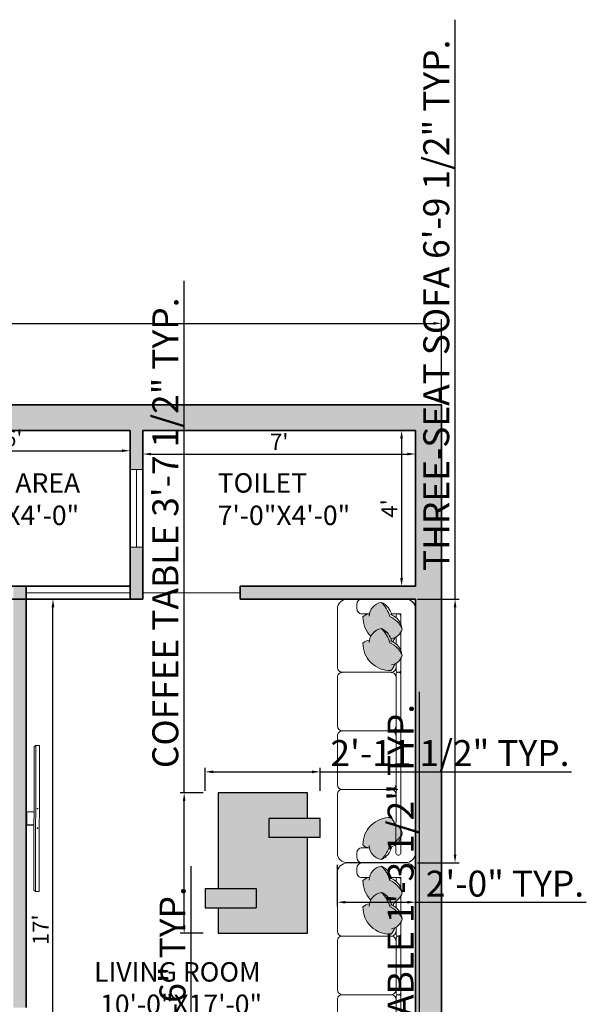
# Model space of a CAD drawing. Units: inches. Extents: x 3259 to 4981, y 1402 to 2026.
# Tile 7 of 11: x 3838 to 4012, y 1722 to 2026. Entities that reach past the tile are written whole.
import ezdxf

# ---------------------------------------------------------------- set-up
doc = ezdxf.new("R2010")
doc.units = ezdxf.units.IN
for name, color, linetype, lineweight in [('A-ANNO-DIMS', 2, 'Continuous', 13), ('A-AREA-IDEN', 7, 'Continuous', 18), ('A-DOOR', 3, 'Continuous', 18), ('A-EQPM', 8, 'Continuous', 18), ('A-FURN', 8, 'Continuous', 13), ('A-GLAZ', 4, 'Continuous', 18), ('A-WALL', 7, 'Continuous', 35), ('A-WALL-PATT', 252, 'Continuous', 13), ('parede', 7, 'Continuous', 30)]:
    doc.layers.add(name, color=color, linetype=linetype, lineweight=lineweight)
doc.styles.get("Standard").update_dxf_attribs({"font": 'arial.ttf'})
doc.dimstyles.new('ISO-25', dxfattribs={"dimtxt": 8, "dimasz": 2.5, "dimexe": 1.25, "dimexo": 0.625, "dimtad": 1, "dimdec": 1, "dimlunit": 3, "dimtxsty": 'Standard', "dimcen": 2.5, "dimclrd": 4, "dimclre": 4, "dimclrt": 1, "dimadec": 0, "dimazin": 0, "dimtfac": 1, "dimtdec": 1, "dimtmove": 0, "dimatfit": 3, "dimfxl": 1, "dimarcsym": 0})

# ---------------------------------------------------------------- blocks, each defined once
blk = doc.blocks.new('SOFA 1')
at = {"transparency": 33554687}
h = blk.add_hatch(color=256, dxfattribs=at)
h.dxf.hatch_style = 1
h.paths.add_polyline_path([(3723.52, 1308.63, 0.147724), (3717.76, 1305.24, 0.310469), (3722.42, 1300.4), (3722.42, 1300.25, 0.156703), (3723.62, 1297.8, 0.425821), (3734.69, 1309.08, 0.121928), (3732.05, 1310.63, 0.233216), (3728.6, 1313.59, 0.213835)])
h = blk.add_hatch(color=256, dxfattribs=at)
h.dxf.hatch_style = 1
h.paths.add_polyline_path([(3769.65, 1307.6, 0.084911), (3767.15, 1309.12, 0.046133), (3766.46, 1311.13), (3759.18, 1311.13, 0.039409), (3758.92, 1310.24, 0.165523), (3756.31, 1309.02, 0.42585), (3767.59, 1297.95, 0.121928), (3769.15, 1300.58, 0.027403), (3769.65, 1300.83)])
h.paths.add_polyline_path([(3765.34, 1313.08), (3760.4, 1313.08, 0.097704), (3759.18, 1311.13), (3766.46, 1311.13, 0.04873)])
h.paths.add_polyline_path([(3763.76, 1314.88, 0.16488), (3760.4, 1313.08), (3765.34, 1313.08, 0.051917)])
h.paths.add_polyline_path([(3771.6, 1305.17, 0.090388), (3769.65, 1307.6), (3769.65, 1300.83, 0.136035), (3771.6, 1302.77)])
h = blk.add_hatch(color=256, dxfattribs=at)
h.dxf.hatch_style = 1
h.paths.add_polyline_path([(3769.16, 1235.96, 0.122267), (3767.6, 1238.61, 0.425972), (3756.32, 1227.54, 0.165563), (3758.93, 1226.32, 0.309481), (3763.76, 1221.69, 0.002677), (3763.83, 1221.72, 0.146094), (3767.16, 1227.43, 0.212433), (3772.1, 1232.48, 0.235342)])
h = blk.add_hatch(color=256, dxfattribs=at)
h.dxf.hatch_style = 1
h.paths.add_polyline_path([(3769.16, 1225.36, 0.122267), (3767.6, 1228.01, 0.425972), (3756.32, 1216.94, 0.165563), (3758.93, 1215.72, 0.309481), (3763.76, 1211.09, 0.002677), (3763.83, 1211.12, 0.146094), (3767.16, 1216.83, 0.212433), (3772.1, 1221.88, 0.235342)])
for p, q in [((3720.45, 1316.13), (3773.58, 1316.13)), ((3777.51, 1312.19), (3777.51, 1213.72))]:
    blk.add_line(p, q, dxfattribs=at)
for points in [[(3716.51, 1312.2), (3716.51, 1291.44)], [(3722.42, 1313.08), (3722.42, 1309.23), (3722.42, 1313.08), (3726.57, 1313.08)], [(3729.85, 1313.08), (3745.25, 1313.08)], [(3746.01, 1312.3), (3746.01, 1288.55)], [(3768.11, 1313.08), (3746.78, 1313.08)], [(3771.6, 1313.08), (3767.75, 1313.08), (3771.6, 1313.08), (3771.6, 1308.93)], [(3769.66, 1287.39), (3769.65, 1312.3)], [(3771.6, 1313.08), (3771.61, 1233.74)], [(3723.21, 1311.13), (3723.93, 1311.13)], [(3731.82, 1311.13), (3745.25, 1311.13)], [(3746.01, 1310.97), (3746.01, 1311.36)], [(3746.01, 1288.54), (3746.01, 1308.23)], [(3768.87, 1311.13), (3746.78, 1311.13)], [(3769.65, 1309.43), (3769.65, 1308.71)], [(3722.42, 1300.39), (3722.42, 1297.33)], [(3720.45, 1295.38), (3718.48, 1295.38)], [(3720.45, 1287.5), (3744.09, 1287.5)], [(3746.02, 1284.63), (3746.02, 1264.94)], [(3747.99, 1286.6), (3767.69, 1286.6)], [(3769.66, 1263.75), (3769.66, 1285.81)], [(3769.66, 1277.18), (3769.66, 1263.75)], [(3746.02, 1260.99), (3746.02, 1241.3)], [(3747.99, 1262.97), (3767.69, 1262.97)], [(3769.66, 1240.12), (3769.66, 1262.18)], [(3770.43, 1262.97), (3770.82, 1262.97)], [(3746.02, 1237.36), (3746.02, 1213.74)], [(3747.99, 1239.33), (3767.69, 1239.33)], [(3769.66, 1235.71), (3769.66, 1238.54)], [(3770.43, 1239.33), (3770.82, 1239.33)], [(3771.61, 1223.14), (3771.61, 1230.47)], [(3769.66, 1225.11), (3769.66, 1227.82)], [(3767.76, 1215.72), (3771.61, 1215.72), (3771.61, 1219.84), (3771.61, 1215.72)], [(3769.66, 1216.5), (3769.66, 1217.22)], [(3753.91, 1211.77), (3753.91, 1213.74)], [(3755.86, 1215.72), (3758.92, 1215.72)], [(3749.97, 1209.8), (3773.58, 1209.8)]]:
    blk.add_lwpolyline(points, close=True, dxfattribs=at)
for points in [[(3717.76, 1305.24, -0.147724), (3723.52, 1308.63, -0.213355), (3728.59, 1313.59, 0.213355), (3723.52, 1308.63, 0.147724), (3717.76, 1305.24, -0.249545), (3722.86, 1309.34, 0.249545), (3717.75, 1305.25, 0.356779), (3723.4, 1300.28, -0.356779), (3717.76, 1305.24)], [(3728.58, 1313.6, -0.306333), (3732.42, 1309.31, 0.306333), (3728.58, 1313.6, 0.306674), (3722.72, 1308.89, -0.306674), (3728.58, 1313.6)], [(3763.76, 1314.88, -0.147724), (3767.15, 1309.12, -0.213355), (3772.1, 1304.05, 0.213355), (3767.15, 1309.12, 0.147724), (3763.76, 1314.88, -0.249545), (3767.86, 1309.77, 0.249545), (3763.77, 1314.89, 0.356779), (3758.8, 1309.23, -0.356779), (3763.76, 1314.88)], [(3734.69, 1309.08, -0.425972), (3723.62, 1297.8, -0.165552), (3722.4, 1300.4, 0.165552), (3723.62, 1297.79, 0.425972), (3734.69, 1309.07, 0.121514), (3732.07, 1310.63, -0.121514), (3734.69, 1309.08)], [(3767.6, 1297.95, -0.425972), (3756.31, 1309.01, -0.165552), (3758.92, 1310.24, 0.165552), (3756.31, 1309.02, 0.425972), (3767.59, 1297.95, 0.121514), (3769.14, 1300.57, -0.121514), (3767.6, 1297.95)], [(3772.11, 1304.06, -0.306333), (3767.83, 1300.22, 0.306333), (3772.11, 1304.06, 0.306674), (3767.4, 1309.91, -0.306674), (3772.11, 1304.06)], [(3770.44, 1286.63, -0.414214), (3769.66, 1287.4, 0.414214), (3770.44, 1286.63, 0.414214), (3769.66, 1285.83, -0.414214), (3770.44, 1286.63)], [(3748.01, 1262.99, -0.414214), (3746.05, 1264.95, 0.414214), (3748.01, 1262.97, 0.414213), (3746.05, 1261.01, -0.414213), (3748.01, 1262.99)], [(3770.44, 1262.99, -0.414214), (3769.66, 1263.77, 0.414214), (3770.44, 1262.99, 0.414214), (3769.66, 1262.19, -0.414214), (3770.44, 1262.99)], [(3770.83, 1262.97, -0.414214), (3771.61, 1262.19, 0.414214), (3770.83, 1262.99, 0.414214), (3771.61, 1263.77, -0.414214), (3770.83, 1262.97)], [(3748.01, 1239.35, -0.414214), (3746.05, 1241.31, 0.414214), (3748.01, 1239.33, 0.414213), (3746.05, 1237.37, -0.414213), (3748.01, 1239.35)], [(3767.7, 1239.33, -0.414214), (3769.66, 1237.37, 0.414214), (3767.7, 1239.35, 0.414214), (3769.66, 1241.31, -0.414214), (3767.7, 1239.33)], [(3770.44, 1239.35, -0.414214), (3769.66, 1240.13, 0.414214), (3770.44, 1239.33, 0.414214), (3769.66, 1238.55, -0.414214), (3770.44, 1239.35)], [(3770.83, 1239.33, -0.414214), (3771.61, 1238.55, 0.414214), (3770.83, 1239.35, 0.414214), (3771.61, 1240.13, -0.414214), (3770.83, 1239.33)], [(3756.32, 1227.54, -0.425972), (3767.6, 1238.61, -0.121514), (3769.16, 1235.98, 0.121514), (3767.6, 1238.61, 0.425972), (3756.32, 1227.54, 0.165552), (3758.93, 1226.32, -0.165552), (3756.32, 1227.54)], [(3772.1, 1232.5, -0.306674), (3767.41, 1226.64, 0.306674), (3772.1, 1232.5, 0.306333), (3767.84, 1236.34, -0.306333), (3772.1, 1232.5)], [(3763.78, 1221.67, 0.249545), (3767.87, 1226.78, -0.249545), (3763.76, 1221.69, -0.356779), (3758.81, 1227.32, 0.356779), (3763.77, 1221.68, 0.147724), (3767.16, 1227.43, 0.213355), (3772.11, 1232.51, -0.213355), (3767.16, 1227.43, -0.147724), (3763.78, 1221.67)], [(3756.32, 1216.94, -0.200233), (3759.49, 1224.76, 0.200233), (3756.32, 1216.94, 0.165552), (3758.93, 1215.72, -0.165552), (3756.32, 1216.94)], [(3772.1, 1221.9, -0.306674), (3767.41, 1216.04, 0.306674), (3772.1, 1221.9, -0.213355), (3767.16, 1216.83, -0.147724), (3763.77, 1211.08, 0.147724), (3767.15, 1216.83, 0.213355), (3772.1, 1221.9)], [(3763.76, 1211.09, -0.356779), (3758.81, 1216.72, 0.356779), (3763.76, 1211.09, 0.249545), (3767.87, 1216.18, -0.249545), (3763.76, 1211.09)]]:
    blk.add_lwpolyline(points, format="xyb", dxfattribs=at)
for points in [[(3722.42, 1311.91, 0.414214), (3723.2, 1311.13, -0.414214)], [(3770.43, 1313.08, 0.414214), (3769.65, 1312.3, -0.414214)], [(3771.6, 1312.3, 0.414214), (3770.82, 1313.08, -0.414214)], [(3716.51, 1297.34, 0.414214), (3718.47, 1295.38, -0.414214)], [(3720.44, 1295.38, 0.414214), (3722.4, 1297.34, -0.414214)], [(3716.51, 1291.45, 0.414212), (3720.44, 1287.52, -0.414212)], [(3746.03, 1288.56, 0.414214), (3747.99, 1286.6, 0.414213), (3746.03, 1284.64, -0.414213), (3747.99, 1286.6, -0.414214)], [(3769.66, 1284.64, 0.414214), (3767.7, 1286.6, 0.414214), (3769.66, 1288.56, -0.414214), (3767.7, 1286.6, -0.414214)], [(3769.66, 1261.01, 0.414214), (3767.7, 1262.97, 0.414214), (3769.66, 1264.93, -0.414214), (3767.7, 1262.97, -0.414214)], [(3772.13, 1221.9, 0.306333), (3767.84, 1225.74, -0.306333)], [(3769.16, 1225.36, 0.071861), (3768.39, 1227.01, -0.071861)], [(3769.66, 1216.52, 0.414214), (3770.44, 1215.74, -0.414214)], [(3770.83, 1215.74, 0.414214), (3771.61, 1216.52, -0.414214)], [(3746.05, 1213.76, 0.414212), (3749.98, 1209.82, -0.414212)], [(3755.87, 1215.72, 0.414214), (3753.91, 1213.76, -0.414214)], [(3755.87, 1209.8, -0.414214), (3753.91, 1211.76, 0.414214)]]:
    blk.add_lwpolyline(points, format="xyb", close=True, dxfattribs=at)
for centre, radius, start, end in [((3720.44, 1312.2), 3.93, 90.0002, 179.9998), ((3720.44, 1312.19), 3.94, 89.9158, 179.9154), ((3773.58, 1312.2), 3.93, 0.0002, 89.9998), ((3773.57, 1312.19), 3.94, 359.9158, 89.9154), ((3745.22, 1312.29), 0.789, 0.8425, 90.8425), ((3745.24, 1311.91), 0.777, 270, 0), ((3745.24, 1311.91), 0.777, 270, 0), ((3746.8, 1312.29), 0.789, 89.1575, 179.1575), ((3746.79, 1311.91), 0.777, 180, 270), ((3746.79, 1311.91), 0.777, 180, 270), ((3768.87, 1312.3), 0.777, 360, 90), ((3768.87, 1311.91), 0.777, 270, 0), ((3744.09, 1309.21), 1.92, 358.766, 90.5111), ((3747.93, 1309.21), 1.92, 89.4889, 181.234), ((3744.08, 1289.48), 1.96, 270, 360), ((3744.08, 1289.48), 1.96, 270, 360), ((3773.58, 1213.73), 3.93, 270.0002, 359.9998), ((3773.59, 1213.73), 3.93, 269.9156, 359.9152)]:
    blk.add_arc(centre, radius, start, end, dxfattribs=at)
blk = doc.blocks.new('Mesa de Centro Nalita')
at = {"layer": 'parede', "ltscale": 0.2}
h = blk.add_hatch(color=256, dxfattribs=at)
h.set_gradient(color1=(95, 72, 63), color2=(161, 128, 114), one_color=1, tint=0.54, name='INVCYLINDER')
h.paths.add_polyline_path([(0.35, -0.35), (0.05, -0.35), (0.05, -0.2), (0.35, -0.2), (0.35, 0), (-0.35, 0), (-0.35, -0.75), (-0.05, -0.75), (-0.05, -0.9), (-0.35, -0.9), (-0.35, -1.1), (0.35, -1.1)])
h = blk.add_hatch(color=256, dxfattribs=at)
h.set_gradient(color1=(95, 72, 63), color2=(161, 128, 114), one_color=1, tint=0.54, name='INVSPHERICAL')
h.paths.add_polyline_path([(0.05, -0.2), (0.05, -0.35), (0.45, -0.35), (0.45, -0.2)])
h = blk.add_hatch(color=256, dxfattribs=at)
h.set_gradient(color1=(95, 72, 63), color2=(161, 128, 114), one_color=1, tint=0.54, name='INVSPHERICAL')
h.paths.add_polyline_path([(-0.05, -0.9), (-0.05, -0.75), (-0.45, -0.75), (-0.45, -0.9)])
for p, q in [((0.35, 0), (-0.35, 0)), ((-0.35, 0), (-0.35, -0.75)), ((0.35, -0.2), (0.35, 0)), ((0.05, -0.35), (0.05, -0.2)), ((0.45, -0.2), (0.05, -0.2)), ((0.45, -0.35), (0.45, -0.2)), ((0.45, -0.35), (0.05, -0.35)), ((0.35, -1.1), (0.35, -0.35)), ((-0.45, -0.75), (-0.05, -0.75)), ((-0.45, -0.75), (-0.45, -0.9)), ((-0.05, -0.75), (-0.05, -0.9)), ((-0.45, -0.9), (-0.05, -0.9)), ((-0.35, -0.9), (-0.35, -1.1)), ((-0.35, -1.1), (0.35, -1.1))]:
    blk.add_line(p, q, dxfattribs=at)
blk = doc.blocks.new('*D44')
at = {"layer": 'A-ANNO-DIMS', "color": 0, "lineweight": -2, "transparency": 16777216}
for p, q in [((3799.66, 1898.49), (3799.66, 1891.66)), ((3871.66, 1898.49), (3871.66, 1891.66)), ((3802.16, 1892.91), (3869.16, 1892.91))]:
    blk.add_line(p, q, dxfattribs=at)
at = {"layer": 'A-ANNO-DIMS', "color": 0, "transparency": 16777216}
for points in [[(3802.16, 1893.33), (3802.16, 1892.5), (3799.66, 1892.91)], [(3869.16, 1893.33), (3869.16, 1892.5), (3871.66, 1892.91)]]:
    blk.add_solid(points, dxfattribs=at)
at = {"layer": 'Defpoints', "color": 0, "transparency": 16777216}
for p in [(3799.66, 1899.12), (3871.66, 1899.12), (3871.66, 1892.91)]:
    blk.add_point(p, dxfattribs=at)
at = {"layer": 'A-ANNO-DIMS', "color": 0, "transparency": 16777216, "insert": (3835.66, 1896.09), "char_height": 5, "attachment_point": 5}
blk.add_mtext("6'", dxfattribs=at)
blk = doc.blocks.new('*D45')
at = {"layer": 'A-ANNO-DIMS', "color": 0, "lineweight": -2, "transparency": 16777216}
for p, q in [((3875.66, 1898.49), (3875.66, 1890.65)), ((3959.66, 1898.49), (3959.66, 1890.65)), ((3878.16, 1891.9), (3957.16, 1891.9))]:
    blk.add_line(p, q, dxfattribs=at)
at = {"layer": 'A-ANNO-DIMS', "color": 0, "transparency": 16777216}
for points in [[(3878.16, 1892.31), (3878.16, 1891.48), (3875.66, 1891.9)], [(3957.16, 1892.31), (3957.16, 1891.48), (3959.66, 1891.9)]]:
    blk.add_solid(points, dxfattribs=at)
at = {"layer": 'Defpoints', "color": 0, "transparency": 16777216}
for p in [(3875.66, 1899.12), (3959.66, 1899.12), (3959.66, 1891.9)]:
    blk.add_point(p, dxfattribs=at)
at = {"layer": 'A-ANNO-DIMS', "color": 0, "transparency": 16777216, "insert": (3917.66, 1895.02), "char_height": 5, "attachment_point": 5}
blk.add_mtext("7'", dxfattribs=at)
blk = doc.blocks.new('*D46')
at = {"layer": 'A-ANNO-DIMS', "color": 0, "lineweight": -2, "transparency": 16777216}
for p, q in [((3959.04, 1899.12), (3954.13, 1899.12)), ((3955.38, 1896.62), (3955.38, 1853.62)), ((3959.04, 1851.12), (3954.13, 1851.12))]:
    blk.add_line(p, q, dxfattribs=at)
at = {"layer": 'A-ANNO-DIMS', "color": 0, "transparency": 16777216}
for points in [[(3954.96, 1896.62), (3955.79, 1896.62), (3955.38, 1899.12)], [(3954.96, 1853.62), (3955.79, 1853.62), (3955.38, 1851.12)]]:
    blk.add_solid(points, dxfattribs=at)
at = {"layer": 'Defpoints', "color": 0, "transparency": 16777216}
for p in [(3959.66, 1899.12), (3955.38, 1851.12), (3959.66, 1851.12)]:
    blk.add_point(p, dxfattribs=at)
at = {"layer": 'A-ANNO-DIMS', "color": 0, "transparency": 16777216, "insert": (3952.25, 1875.12), "char_height": 5, "attachment_point": 5, "rotation": 90}
blk.add_mtext("4'", dxfattribs=at)
blk = doc.blocks.new('*D56')
at = {"layer": 'A-ANNO-DIMS', "color": 0, "lineweight": -2, "transparency": 16777216}
for p, q in [((3840.29, 1847.12), (3849.16, 1847.12)), ((3847.91, 1645.62), (3847.91, 1844.62)), ((3840.29, 1643.12), (3849.16, 1643.12))]:
    blk.add_line(p, q, dxfattribs=at)
at = {"layer": 'A-ANNO-DIMS', "color": 0, "transparency": 16777216}
for points in [[(3847.49, 1844.62), (3848.33, 1844.62), (3847.91, 1847.12)], [(3847.49, 1645.62), (3848.33, 1645.62), (3847.91, 1643.12)]]:
    blk.add_solid(points, dxfattribs=at)
at = {"layer": 'Defpoints', "color": 0, "transparency": 16777216}
for p in [(3839.66, 1847.12), (3847.91, 1847.12), (3839.66, 1643.12)]:
    blk.add_point(p, dxfattribs=at)
at = {"layer": 'A-ANNO-DIMS', "color": 0, "transparency": 16777216, "insert": (3844.77, 1745.12), "char_height": 5, "attachment_point": 5, "rotation": 90}
blk.add_mtext("17'", dxfattribs=at)
blk = doc.blocks.new('SOFA-3SEAT')
at = {"transparency": 33554687}
h = blk.add_hatch(color=256, dxfattribs=at)
h.dxf.hatch_style = 1
h.paths.add_polyline_path([(17.7, 69.38, -0.122267), (16.5, 67.36, -0.425972), (7.88, 75.82, -0.165563), (9.87, 76.76, -0.309481), (13.57, 80.3, -0.002677), (13.62, 80.27, -0.146094), (16.16, 75.9, -0.212433), (19.95, 72.05, -0.235342)])
h = blk.add_hatch(color=256, dxfattribs=at)
h.dxf.hatch_style = 1
h.paths.add_polyline_path([(17.7, 61.28, -0.122267), (16.5, 59.26, -0.425972), (7.88, 67.72, -0.165563), (9.87, 68.65, -0.309481), (13.57, 72.19, -0.002677), (13.62, 72.17, -0.146094), (16.16, 67.8, -0.212433), (19.95, 63.95, -0.235342)])
h = blk.add_hatch(color=256, dxfattribs=at)
h.dxf.hatch_style = 1
h.paths.add_polyline_path([(18.07, 6.52, -0.084911), (16.16, 5.36, -0.046133), (15.63, 3.82), (10.07, 3.82, -0.039409), (9.87, 4.51, -0.165523), (7.87, 5.44, -0.42585), (16.5, 13.9, -0.121928), (17.69, 11.88, -0.027403), (18.07, 11.69)])
h.paths.add_polyline_path([(14.77, 2.33), (11, 2.33, -0.097704), (10.07, 3.82), (15.63, 3.82, -0.04873)])
h.paths.add_polyline_path([(13.57, 0.96, -0.16488), (11, 2.33), (14.77, 2.33, -0.051917)])
h.paths.add_polyline_path([(19.56, 8.38, -0.090388), (18.07, 6.52), (18.07, 11.69, -0.136035), (19.56, 10.21)])
blk.add_line((24.08, 3.01), (24.08, 78.28), dxfattribs=at)
blk.add_line((18.66, 2.33), (18.96, 2.33))
for points in [[(0.03, 78.26, -0.414212), (3.03, 81.26, 0.414212)], [(7.54, 81.28, 0.414214), (6.04, 79.78, -0.414214)], [(7.54, 76.76, -0.414214), (6.04, 78.26, 0.414214)], [(18.08, 76.15, -0.414214), (18.67, 76.74, 0.414214)], [(18.97, 76.74, -0.414214), (19.57, 76.15, 0.414214)], [(19.96, 72.03, -0.306333), (16.68, 69.1, 0.306333)], [(17.69, 69.39, -0.071861), (17.1, 68.12, 0.071861)], [(18.08, 42.14, -0.414214), (16.58, 40.64, -0.414214), (18.08, 39.14, 0.414214), (16.58, 40.64, 0.414214)], [(0.02, 21.07, -0.414214), (1.52, 22.57, -0.414213), (0.02, 24.07, 0.414213), (1.52, 22.57, 0.414214)], [(18.08, 24.07, -0.414214), (16.58, 22.57, -0.414214), (18.08, 21.07, 0.414214), (16.58, 22.57, 0.414214)], [(7.54, 4.54, 0.414214), (6.04, 3.04, -0.414214)], [(0, 2.93, 0.439287), (3.02, 0.02, -0.439287)], [(7.54, 0.02, -0.414214), (6.04, 1.52, 0.414214)], [(18.66, 2.33, -0.414214), (18.07, 2.93, 0.414214)], [(19.56, 2.93, -0.414214), (18.96, 2.33, 0.414214)]]:
    blk.add_lwpolyline(points, format="xyb", close=True, dxfattribs=at)
for points in [[(3.02, 81.28), (21.07, 81.28)], [(6.04, 79.77), (6.04, 78.27)], [(0.01, 60.21), (0.01, 78.27)], [(7.53, 76.76), (9.87, 76.76)], [(16.62, 76.76), (19.57, 76.76), (19.57, 73.6), (19.57, 76.76)], [(18.08, 76.16), (18.08, 75.61)], [(19.57, 71.08), (19.57, 65.48)], [(18.08, 69.58), (18.08, 67.5)], [(18.08, 61.47), (18.08, 59.31)], [(19.56, 2.93), (19.57, 62.98)], [(1.52, 58.71), (16.57, 58.71)], [(18.08, 58.1), (18.08, 41.24)], [(18.66, 58.71), (18.96, 58.71)], [(0.01, 42.15), (0.01, 57.2)], [(1.52, 40.64), (16.57, 40.64)], [(18.08, 29.77), (18.08, 40.04)], [(18.08, 40.04), (18.08, 23.17)], [(18.66, 40.64), (18.96, 40.64)], [(0.01, 24.08), (0.01, 39.13)], [(1.52, 22.57), (16.57, 22.57)], [(18.08, 21.97), (18.07, 2.93)], [(0, 2.93), (0, 21.08)], [(0, 3.95), (0, 3.64)], [(7.53, 4.54), (9.87, 4.54)], [(18.07, 5.12), (18.07, 5.67)], [(3.02, 0.02), (21.07, 0.02)], [(6.04, 1.52), (6.04, 3.03)]]:
    blk.add_lwpolyline(points, close=True, dxfattribs=at)
for points in [[(13.57, 80.3, 0.356779), (9.78, 75.99, -0.356779), (13.57, 80.3, -0.249545), (16.71, 76.4, 0.249545), (13.57, 80.3)], [(19.94, 72.03, 0.306674), (16.36, 76.51, -0.306674), (19.94, 72.03, 0.213355), (16.16, 75.9, 0.147724), (13.58, 80.3, -0.147724), (16.16, 75.91, -0.213355), (19.94, 72.03)], [(7.88, 75.82, 0.200233), (10.31, 69.84, -0.200233), (7.88, 75.82, -0.165552), (9.87, 76.76, 0.165552), (7.88, 75.82)], [(13.58, 72.21, -0.249545), (16.71, 68.3, 0.249545), (13.57, 72.19, 0.356779), (9.78, 67.89, -0.356779), (13.58, 72.2, -0.147724), (16.16, 67.8, -0.213355), (19.95, 63.92, 0.213355), (16.16, 67.8, 0.147724), (13.58, 72.21)], [(7.88, 67.72, 0.425972), (16.5, 59.26, 0.121514), (17.69, 61.27, -0.121514), (16.5, 59.26, -0.425972), (7.88, 67.72, -0.165552), (9.87, 68.65, 0.165552), (7.88, 67.72)], [(19.94, 63.93, 0.306674), (16.36, 68.41, -0.306674), (19.94, 63.93, -0.306333), (16.68, 61, 0.306333), (19.94, 63.93)], [(1.52, 58.69, 0.414214), (0.03, 57.19, -0.414214), (1.52, 58.71, -0.414213), (0.03, 60.21, 0.414213), (1.52, 58.69)], [(16.58, 58.71, 0.414214), (18.08, 60.21, -0.414214), (16.58, 58.69, -0.414214), (18.08, 57.19, 0.414214), (16.58, 58.71)], [(18.67, 58.69, 0.414214), (18.08, 58.1, -0.414214), (18.67, 58.71, -0.414214), (18.08, 59.3, 0.414214), (18.67, 58.69)], [(18.97, 58.71, 0.414214), (19.57, 59.3, -0.414214), (18.97, 58.69, -0.414214), (19.57, 58.1, 0.414214), (18.97, 58.71)], [(1.52, 40.62, 0.414214), (0.03, 39.12, -0.414214), (1.52, 40.64, -0.414213), (0.03, 42.14, 0.414213), (1.52, 40.62)], [(18.67, 40.62, 0.414214), (18.08, 40.03, -0.414214), (18.67, 40.62, -0.414214), (18.08, 41.23, 0.414214), (18.67, 40.62)], [(18.97, 40.64, 0.414214), (19.57, 41.23, -0.414214), (18.97, 40.62, -0.414214), (19.57, 40.03, 0.414214), (18.97, 40.64)], [(18.67, 22.55, 0.414214), (18.08, 21.96, -0.414214), (18.67, 22.55, -0.414214), (18.08, 23.17, 0.414214), (18.67, 22.55)], [(16.5, 13.9, 0.425972), (7.87, 5.44, 0.165552), (9.87, 4.51, -0.165552), (7.87, 5.44, -0.425972), (16.5, 13.9, -0.121514), (17.68, 11.89, 0.121514), (16.5, 13.9)], [(19.95, 9.23, 0.306333), (16.68, 12.16, -0.306333), (19.95, 9.23, -0.306674), (16.35, 4.75, 0.306674), (19.95, 9.23)], [(13.57, 0.96, 0.147724), (16.16, 5.36, 0.213355), (19.94, 9.23, -0.213355), (16.16, 5.36, -0.147724), (13.57, 0.96, 0.249545), (16.7, 4.86, -0.249545), (13.57, 0.95, -0.356779), (9.77, 5.27, 0.356779), (13.57, 0.96)]]:
    blk.add_lwpolyline(points, format="xyb", dxfattribs=at)
for centre, radius, start, end in [((21.08, 78.28), 3, 0.0848, 90.0844), ((21.07, 78.27), 3.01, 0.0002, 89.9998), ((21.07, 3.01), 3.01, 270.0002, 359.9998), ((21.07, 3.01), 3.01, 270.0846, 0.0842)]:
    blk.add_arc(centre, radius, start, end, dxfattribs=at)
blk = doc.blocks.new('*D152')
at = {"layer": 'A-ANNO-DIMS', "color": 4, "lineweight": -2, "transparency": 16777216}
for p, q in [((3890.55, 1617.63), (3890.55, 1764.73)), ((3886.68, 1617.63), (3891.8, 1617.63)), ((3890.55, 1590.15), (3890.55, 1615.13)), ((3886.68, 1587.65), (3891.8, 1587.65))]:
    blk.add_line(p, q, dxfattribs=at)
at = {"layer": 'A-ANNO-DIMS', "color": 4, "transparency": 16777216}
for points in [[(3890.13, 1615.13), (3890.96, 1615.13), (3890.55, 1617.63)], [(3890.13, 1590.15), (3890.96, 1590.15), (3890.55, 1587.65)]]:
    blk.add_solid(points, dxfattribs=at)
at = {"layer": 'Defpoints', "color": 0, "transparency": 16777216}
for p in [(3886.05, 1617.63), (3890.55, 1617.63), (3886.05, 1587.65)]:
    blk.add_point(p, dxfattribs=at)
at = {"layer": 'A-ANNO-DIMS', "color": 1, "transparency": 16777216, "insert": (3885.79, 1692.43), "char_height": 8, "attachment_point": 5, "rotation": 90}
blk.add_mtext('TERRACE CHAIR 2\'-6" TYP.', dxfattribs=at)
blk = doc.blocks.new('*D160')
at = {"layer": 'A-ANNO-DIMS', "color": 4, "lineweight": -2, "transparency": 16777216}
for p, q in [((3960.87, 1679.69), (3960.87, 1818.51)), ((3959.13, 1679.69), (3962.12, 1679.69)), ((3960.87, 1666.44), (3960.87, 1677.19)), ((3959.13, 1663.94), (3962.12, 1663.94))]:
    blk.add_line(p, q, dxfattribs=at)
at = {"layer": 'A-ANNO-DIMS', "color": 4, "transparency": 16777216}
for points in [[(3960.45, 1677.19), (3961.28, 1677.19), (3960.87, 1679.69)], [(3960.45, 1666.44), (3961.28, 1666.44), (3960.87, 1663.94)]]:
    blk.add_solid(points, dxfattribs=at)
at = {"layer": 'Defpoints', "color": 0, "transparency": 16777216}
for p in [(3958.51, 1679.69), (3960.87, 1679.69), (3958.51, 1663.94)]:
    blk.add_point(p, dxfattribs=at)
at = {"layer": 'A-ANNO-DIMS', "color": 1, "transparency": 16777216, "insert": (3956.1, 1750.35), "char_height": 8, "attachment_point": 5, "rotation": 90}
blk.add_mtext('SIDE TABLE 1\'-3 1/2" TYP.', dxfattribs=at)
blk = doc.blocks.new('*D162')
at = {"layer": 'A-ANNO-DIMS', "color": 4, "lineweight": -2, "transparency": 16777216}
for p, q in [((3888.35, 1787.34), (3888.35, 1945.34)), ((3894.22, 1787.34), (3887.1, 1787.34)), ((3888.35, 1746.53), (3888.35, 1784.84)), ((3894.22, 1744.03), (3887.1, 1744.03))]:
    blk.add_line(p, q, dxfattribs=at)
at = {"layer": 'A-ANNO-DIMS', "color": 4, "transparency": 16777216}
for points in [[(3887.94, 1784.84), (3888.77, 1784.84), (3888.35, 1787.34)], [(3887.94, 1746.53), (3888.77, 1746.53), (3888.35, 1744.03)]]:
    blk.add_solid(points, dxfattribs=at)
at = {"layer": 'Defpoints', "color": 0, "transparency": 16777216}
for p in [(3888.35, 1787.34), (3894.85, 1787.34), (3894.85, 1744.03)]:
    blk.add_point(p, dxfattribs=at)
at = {"layer": 'A-ANNO-DIMS', "color": 1, "transparency": 16777216, "insert": (3883.59, 1867.59), "char_height": 8, "attachment_point": 5, "rotation": 90}
blk.add_mtext('COFFEE TABLE 3\'-7 1/2" TYP.', dxfattribs=at)
blk = doc.blocks.new('*D163')
at = {"layer": 'A-ANNO-DIMS', "color": 4, "lineweight": -2, "transparency": 16777216}
for p, q in [((3894.85, 1787.96), (3894.85, 1795.08)), ((3897.35, 1793.83), (3927.78, 1793.83)), ((3930.28, 1787.96), (3930.28, 1795.08)), ((3930.28, 1793.83), (4007.79, 1793.83))]:
    blk.add_line(p, q, dxfattribs=at)
at = {"layer": 'A-ANNO-DIMS', "color": 4, "transparency": 16777216}
for points in [[(3897.35, 1794.25), (3897.35, 1793.41), (3894.85, 1793.83)], [(3927.78, 1794.25), (3927.78, 1793.41), (3930.28, 1793.83)]]:
    blk.add_solid(points, dxfattribs=at)
at = {"layer": 'Defpoints', "color": 0, "transparency": 16777216}
for p in [(3930.28, 1793.83), (3894.85, 1787.34), (3930.28, 1787.34)]:
    blk.add_point(p, dxfattribs=at)
at = {"layer": 'A-ANNO-DIMS', "color": 1, "transparency": 16777216, "insert": (3970.29, 1798.59), "char_height": 8, "attachment_point": 5}
blk.add_mtext('2\'-11 1/2" TYP.', dxfattribs=at)
blk = doc.blocks.new('*D166')
at = {"layer": 'A-ANNO-DIMS', "color": 4, "lineweight": -2, "transparency": 16777216}
for p, q in [((3971.86, 1847.12), (3971.86, 2025.91)), ((3960.29, 1847.12), (3973.11, 1847.12)), ((3971.86, 1768.31), (3971.86, 1844.62)), ((3960.29, 1765.81), (3973.11, 1765.81))]:
    blk.add_line(p, q, dxfattribs=at)
at = {"layer": 'A-ANNO-DIMS', "color": 4, "transparency": 16777216}
for points in [[(3971.45, 1844.62), (3972.28, 1844.62), (3971.86, 1847.12)], [(3971.45, 1768.31), (3972.28, 1768.31), (3971.86, 1765.81)]]:
    blk.add_solid(points, dxfattribs=at)
at = {"layer": 'Defpoints', "color": 0, "transparency": 16777216}
for p in [(3959.67, 1847.12), (3971.86, 1847.12), (3959.67, 1765.81)]:
    blk.add_point(p, dxfattribs=at)
at = {"layer": 'A-ANNO-DIMS', "color": 1, "transparency": 16777216, "insert": (3967.1, 1937.77), "char_height": 8, "attachment_point": 5, "rotation": 90}
blk.add_mtext('THREE-SEAT SOFA 6\'-9 1/2" TYP.', dxfattribs=at)
blk = doc.blocks.new('*D167')
at = {"layer": 'A-ANNO-DIMS', "color": 4, "lineweight": -2, "transparency": 16777216}
for p, q in [((3935.57, 1765.19), (3935.57, 1752.36)), ((3959.67, 1765.19), (3959.67, 1752.36)), ((3938.07, 1753.61), (3957.17, 1753.61)), ((3959.67, 1753.61), (4012.32, 1753.61))]:
    blk.add_line(p, q, dxfattribs=at)
at = {"layer": 'A-ANNO-DIMS', "color": 4, "transparency": 16777216}
for points in [[(3938.07, 1754.03), (3938.07, 1753.2), (3935.57, 1753.61)], [(3957.17, 1754.03), (3957.17, 1753.2), (3959.67, 1753.61)]]:
    blk.add_solid(points, dxfattribs=at)
at = {"layer": 'Defpoints', "color": 0, "transparency": 16777216}
for p in [(3935.57, 1765.81), (3959.67, 1765.81), (3959.67, 1753.61)]:
    blk.add_point(p, dxfattribs=at)
at = {"layer": 'A-ANNO-DIMS', "color": 1, "transparency": 16777216, "insert": (3987.24, 1758.32), "char_height": 8, "attachment_point": 5}
blk.add_mtext('2\'-0" TYP.', dxfattribs=at)
blk = doc.blocks.new('*D186')
at = {"layer": 'A-ANNO-DIMS', "color": 4, "lineweight": -2, "transparency": 16777216}
for p, q in [((3667.66, 1907.74), (3667.66, 1933.47)), ((3670.16, 1932.22), (3965.16, 1932.22)), ((3967.66, 1907.74), (3967.66, 1933.47))]:
    blk.add_line(p, q, dxfattribs=at)
at = {"layer": 'A-ANNO-DIMS', "color": 4, "transparency": 16777216}
for points in [[(3670.16, 1932.63), (3670.16, 1931.8), (3667.66, 1932.22)], [(3965.16, 1932.63), (3965.16, 1931.8), (3967.66, 1932.22)]]:
    blk.add_solid(points, dxfattribs=at)
at = {"layer": 'Defpoints', "color": 0, "transparency": 16777216}
for p in [(3967.66, 1932.22), (3667.66, 1907.12), (3967.66, 1907.12)]:
    blk.add_point(p, dxfattribs=at)
at = {"layer": 'A-ANNO-DIMS', "color": 1, "transparency": 16777216, "insert": (3817.66, 1936.93), "char_height": 8, "attachment_point": 5}
blk.add_mtext('25\'-0"', dxfattribs=at)

msp = doc.modelspace()

# ---------------------------------------------------------------- hatches: boundary and pattern name
at = {"layer": 'A-WALL-PATT'}
h = msp.add_hatch(color=256, dxfattribs=at)
h.dxf.hatch_style = 1
h.paths.add_polyline_path([(3839.66, 1851.12), (3835.66, 1851.12), (3835.66, 1721.12), (3839.66, 1721.12), (3839.66, 1777.43), (3839.65, 1777.43), (3839.65, 1777.47), (3839.66, 1777.47), (3839.66, 1781.5), (3839.66, 1781.5), (3839.66, 1781.55)], flags=17)
h.paths.add_polyline_path([(3799.66, 1863.12), (3795.66, 1863.12), (3795.66, 1851.12), (3711.66, 1851.12), (3711.66, 1847.12), (3749.49, 1847.12), (3749.49, 1847.13), (3749.54, 1847.13), (3749.54, 1847.12), (3753.57, 1847.12), (3753.57, 1847.12), (3753.61, 1847.12), (3799.66, 1847.12)], flags=17)
h.paths.add_polyline_path([(3875.66, 1863.12), (3871.66, 1863.12), (3871.66, 1847.12), (3875.66, 1847.12)], flags=17)
h.paths.add_polyline_path([(3967.66, 1907.12), (3667.66, 1907.12), (3667.66, 1579.12), (3839.66, 1579.12), (3839.66, 1587.12), (3835.66, 1587.12), (3835.66, 1583.12), (3675.66, 1583.12), (3675.66, 1721.12), (3799.66, 1721.12), (3799.66, 1725.12), (3675.66, 1725.12), (3675.66, 1899.12), (3711.66, 1899.12), (3711.66, 1881.12), (3715.66, 1881.12), (3715.66, 1899.12), (3795.66, 1899.12), (3795.66, 1887.12), (3799.66, 1887.12), (3799.66, 1899.12), (3871.66, 1899.12), (3871.66, 1887.12), (3875.66, 1887.12), (3875.66, 1899.12), (3959.66, 1899.12), (3959.66, 1851.12), (3905.66, 1851.12), (3905.66, 1847.12), (3959.66, 1847.12), (3959.66, 1643.12), (3941.66, 1643.12), (3941.66, 1639.12), (3967.66, 1639.12)])
h.paths.add_polyline_path([(3839.66, 1667.12), (3835.66, 1667.12), (3835.66, 1635.12), (3839.66, 1635.12), (3839.66, 1639.12), (3857.66, 1639.12), (3857.66, 1643.12), (3839.66, 1643.12)], flags=17)

# ---------------------------------------------------------------- linework, layer by layer
at = {"layer": 'A-DOOR'}
for p, q in [((3839.66, 1849.12), (3871.66, 1849.12)), ((3905.66, 1849.12), (3875.66, 1849.12))]:
    msp.add_line(p, q, dxfattribs=at)
at = {"layer": 'A-EQPM'}
for p, q in [((3842.01, 1757.35), (3842.1, 1801.61)), ((3842.58, 1802.01), (3842.1, 1801.61)), ((3839.66, 1781.55), (3842.06, 1781.54)), ((3839.66, 1781.5), (3839.66, 1781.55)), ((3839.66, 1781.5), (3842.06, 1781.49)), ((3839.89, 1777.47), (3839.9, 1781.5)), ((3839.65, 1777.47), (3842.05, 1777.47)), ((3839.65, 1777.43), (3839.65, 1777.47)), ((3839.65, 1777.43), (3842.05, 1777.42)), ((3842.49, 1756.95), (3842.01, 1757.35))]:
    msp.add_line(p, q, dxfattribs=at)
msp.add_lwpolyline([(3843.69, 1756.95), (3843.78, 1802.01), (3842.58, 1802.01), (3842.49, 1756.95), (3843.69, 1756.95)], dxfattribs=at)
for centre in [(3843.14, 1782.48), (3843.13, 1776.48)]:
    msp.add_circle(centre, 0.0959, dxfattribs=at)
at = {"layer": 'A-GLAZ'}
for p, q in [((3871.66, 1887.12), (3875.66, 1887.12)), ((3873.66, 1887.12), (3873.66, 1863.12)), ((3871.66, 1863.12), (3875.66, 1863.12))]:
    msp.add_line(p, q, dxfattribs=at)
at = {"layer": 'A-WALL'}
for p, q in [((3799.66, 1899.12), (3871.66, 1899.12)), ((3871.66, 1899.12), (3871.66, 1847.12)), ((3875.66, 1899.12), (3959.66, 1899.12)), ((3875.66, 1899.12), (3875.66, 1847.12)), ((3959.66, 1899.12), (3959.66, 1851.12)), ((3799.66, 1851.12), (3871.66, 1851.12)), ((3839.66, 1721.12), (3839.66, 1851.12)), ((3905.66, 1851.12), (3959.66, 1851.12)), ((3905.66, 1851.12), (3905.66, 1847.12)), ((3711.66, 1847.12), (3871.66, 1847.12)), ((3871.66, 1847.12), (3875.66, 1847.12)), ((3905.66, 1847.12), (3959.66, 1847.12)), ((3959.66, 1847.12), (3959.66, 1643.12))]:
    msp.add_line(p, q, dxfattribs=at)
msp.add_lwpolyline([(3959.66, 1475.12), (3667.66, 1475.12), (3667.66, 1907.12), (3967.66, 1907.12), (3967.66, 1475.12), (3959.66, 1475.12)], dxfattribs=at)

# ---------------------------------------------------------------- block references
at = {"layer": 'A-FURN'}
msp.add_blockref('SOFA-3SEAT', (3935.58, 1765.84), dxfattribs=at)
at = {"layer": 'A-FURN', "xscale": 39.3701, "yscale": 39.3701, "zscale": 39.3701}
msp.add_blockref('Mesa de Centro Nalita', (3912.57, 1787.34), dxfattribs=at)
at = {"layer": 'A-FURN', "xscale": -0.7644053585719659, "yscale": 0.7644053585719659, "zscale": 0.7644053585719659, "rotation": 180}
msp.add_blockref('SOFA 1', (1072.11, 2690.51), dxfattribs=at)

# ---------------------------------------------------------------- texts
at = {"layer": 'A-AREA-IDEN', "char_height": 6, "attachment_point": 1}
for s, insert in [('WASH AREA\\P  6\'-0"X4\'-0"', (3811.47, 1885.99)), ('TOILET\\P7\'-0"X4\'-0"', (3898.69, 1885.99)), ('LIVING ROOM\\P 10\'-0"X17\'-0"', (3860.6, 1735.12))]:
    msp.add_mtext_dynamic_manual_height_columns(s, width=127.3061, gutter_width=12.5, heights=[0], dxfattribs=dict(at, insert=insert))

# ---------------------------------------------------------------- dimensions: what is measured, and where the dimension line sits
at = {"layer": 'A-ANNO-DIMS'}
for base, p1, p2, text, picture, middle in [((3971.86, 1847.12), (3959.67, 1765.81), (3959.67, 1847.12), 'THREE-SEAT SOFA <> TYP.', '*D166', (3967.1, 1937.77)), ((3888.35, 1787.34), (3894.85, 1744.03), (3894.85, 1787.34), 'COFFEE TABLE <> TYP.', '*D162', (3883.59, 1867.59)), ((3960.8677, 1679.6915), (3958.5055, 1663.9434), (3958.5055, 1679.6915), 'SIDE TABLE <> TYP.', '*D160', (3956.1035, 1750.3499)), ((3890.55, 1617.63), (3886.05, 1587.65), (3886.05, 1617.63), 'TERRACE CHAIR <> TYP.', '*D152', (3885.79, 1692.43))]:
    dim = msp.add_linear_dim(base=base, p1=p1, p2=p2, angle=90, text=text, dimstyle='ISO-25', override={"dimdec": 1, "dimlfac": 1, "dimrnd": 0, "dimzin": 1, "dimdsep": 46, "dimlunit": 4, "dimfrac": 2}, dxfattribs=at)
    dim.commit()
    dim.dimension.update_dxf_attribs({"geometry": picture, "text_midpoint": middle})
for base, p1, p2, override, picture, middle in [((3967.66, 1932.22), (3667.66, 1907.12), (3967.66, 1907.12), {"dimdec": 1, "dimlfac": 1, "dimrnd": 0, "dimzin": 1, "dimdsep": 46, "dimlunit": 4, "dimfrac": 2}, '*D186', (3817.66, 1936.93)), ((3871.66, 1892.91), (3799.66, 1899.12), (3871.66, 1899.12), {"dimtxt": 5, "dimclrd": 0, "dimclre": 0, "dimclrt": 0}, '*D44', (3835.66, 1896.09)), ((3959.66, 1891.9), (3875.66, 1899.12), (3959.66, 1899.12), {"dimtxt": 5, "dimclrd": 0, "dimclre": 0, "dimclrt": 0}, '*D45', (3917.66, 1895.02))]:
    dim = msp.add_linear_dim(base=base, p1=p1, p2=p2, dimstyle='ISO-25', override=override, dxfattribs=at)
    dim.commit()
    dim.dimension.update_dxf_attribs({"geometry": picture, "text_midpoint": middle})
for base, p1, p2, picture, middle in [((3955.38, 1851.12), (3959.66, 1899.12), (3959.66, 1851.12), '*D46', (3952.25, 1875.12)), ((3847.91, 1847.12), (3839.66, 1643.12), (3839.66, 1847.12), '*D56', (3844.77, 1745.12))]:
    dim = msp.add_linear_dim(base=base, p1=p1, p2=p2, angle=90, dimstyle='ISO-25', override={"dimtxt": 5, "dimclrd": 0, "dimclre": 0, "dimclrt": 0}, dxfattribs=at)
    dim.commit()
    dim.dimension.update_dxf_attribs({"geometry": picture, "text_midpoint": middle})
for base, p1, p2, picture, middle in [((3930.28, 1793.83), (3894.85, 1787.34), (3930.28, 1787.34), '*D163', (3970.29, 1798.59)), ((3959.67, 1753.61), (3935.57, 1765.81), (3959.67, 1765.81), '*D167', (3987.24, 1758.32))]:
    dim = msp.add_linear_dim(base=base, p1=p1, p2=p2, text='<> TYP.', dimstyle='ISO-25', override={"dimdec": 1, "dimlfac": 1, "dimrnd": 0, "dimzin": 1, "dimdsep": 46, "dimlunit": 4, "dimfrac": 2}, dxfattribs=at)
    dim.commit()
    dim.dimension.update_dxf_attribs({"geometry": picture, "text_midpoint": middle})

doc.saveas('drawing.dxf')
